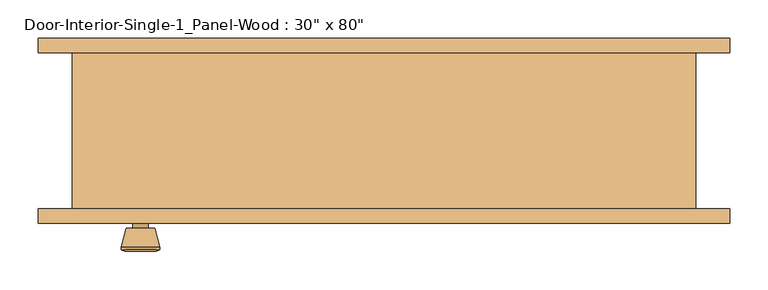
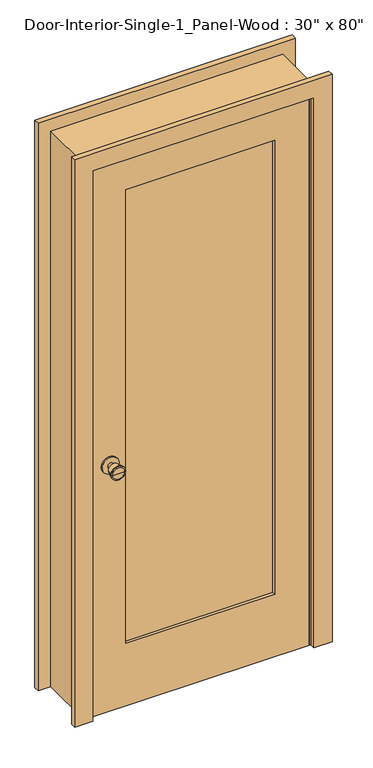
"""IFC4 building model written with IfcOpenShell, lengths in millimetres: door geometry."""

from ifc_helpers import new_model, si_unit, point, frame, frame_2d, origin, place, context, project, spatial, polyline, circle_curve, trimmed, segment, composite_curve, outline, extrude, faceted_brep, source, transform, mapped, element, save
from ifc_brep_helpers import plane_surface, cylinder_surface, revolved_surface, advanced_brep


def door_975671f7(model_context):
    return source(origin(), model_context, "Body", "SolidModel", [
        advanced_brep(
        [(-317.5, -57.5, 914.4), (-327.5, -57.5, 914.4), (-307.5, -57.5, 914.4), (-297.0241324, -8.5, 914.4), (-337.9758676, -8.5, 914.4), (-317.5, -8.5, 914.4), (-292.5, -10.3278681, 914.4), (-342.5, -10.3278681, 914.4), (-292.5, -13.7915463, 914.4), (-342.5, -13.7915463, 914.4), (-298.863764, -38.5, 914.4), (-336.136236, -38.5, 914.4), (-307.5, -38.5, 914.4), (-327.5, -38.5, 914.4)],
        [
            (0, 1),
            (1, 2, circle_curve(frame((-317.5, -57.5, 914.4), z_axis=(0.0, -1.0, 0.0), x_axis=(-1.0, 0.0, 0.0)), 10.0)),
            (2, 0),
            (2, 1, circle_curve(frame((-317.5, -57.5, 914.4), z_axis=(0.0, -1.0, 0.0), x_axis=(-1.0, 0.0, 0.0)), 10.0)),
            (3, 4, circle_curve(frame((-317.5, -8.5, 914.4), z_axis=(0.0, 1.0, 0.0), x_axis=(-1.0, 0.0, 0.0)), 20.4758676)),
            (4, 5),
            (5, 3),
            (4, 3, circle_curve(frame((-317.5, -8.5, 914.4), z_axis=(0.0, 1.0, 0.0), x_axis=(-1.0, 0.0, 0.0)), 20.4758676)),
            (6, 7, circle_curve(frame((-317.5, -10.3278681, 914.4), z_axis=(0.0, 1.0, 0.0), x_axis=(-1.0, 0.0, 0.0)), 25.0)),
            (7, 4),
            (3, 6),
            (7, 6, circle_curve(frame((-317.5, -10.3278681, 914.4), z_axis=(0.0, 1.0, 0.0), x_axis=(-1.0, 0.0, 0.0)), 25.0)),
            (8, 9, circle_curve(frame((-317.5, -13.7915463, 914.4), z_axis=(0.0, 1.0, 0.0), x_axis=(-1.0, 0.0, 0.0)), 25.0)),
            (9, 7),
            (6, 8),
            (9, 8, circle_curve(frame((-317.5, -13.7915463, 914.4), z_axis=(0.0, 1.0, 0.0), x_axis=(-1.0, 0.0, 0.0)), 25.0)),
            (10, 11, circle_curve(frame((-317.5, -38.5, 914.4), z_axis=(0.0, 1.0, 0.0), x_axis=(-1.0, 0.0, 0.0)), 18.636236)),
            (11, 9),
            (8, 10),
            (11, 10, circle_curve(frame((-317.5, -38.5, 914.4), z_axis=(0.0, 1.0, 0.0), x_axis=(-1.0, 0.0, 0.0)), 18.636236)),
            (12, 13, circle_curve(frame((-317.5, -38.5, 914.4), z_axis=(0.0, 1.0, 0.0), x_axis=(-1.0, 0.0, 0.0)), 10.0)),
            (13, 11),
            (10, 12),
            (13, 12, circle_curve(frame((-317.5, -38.5, 914.4), z_axis=(0.0, 1.0, 0.0), x_axis=(-1.0, 0.0, 0.0)), 10.0)),
            (1, 13),
            (12, 2),
        ],
        [
            plane_surface(frame((-317.5, -57.5, 914.4), z_axis=(0.0, -1.0, 0.0), x_axis=(-1.0, 0.0, 0.0))),
            plane_surface(frame((-317.5, -8.5, 914.4), z_axis=(0.0, 1.0, 0.0), x_axis=(-1.0, 0.0, 0.0))),
            revolved_surface(polyline([(-337.9758676, -8.5, 914.4), (-342.5, -10.3278681, 914.4)]), (-317.5, -57.5, 914.4), (0.0, -1.0, 0.0)),
            cylinder_surface(frame((-317.5, -57.5, 914.4), z_axis=(0.0, -1.0, 0.0), x_axis=(-1.0, 0.0, 0.0)), 25.0),
            revolved_surface(polyline([(-342.5, -13.7915463, 914.4), (-336.136236, -38.5, 914.4)]), (-317.5, -57.5, 914.4), (0.0, -1.0, 0.0)),
            plane_surface(frame((-317.5, -38.5, 914.4), z_axis=(0.0, -1.0, 0.0), x_axis=(-1.0, 0.0, 0.0))),
            cylinder_surface(frame((-317.5, -57.5, 914.4), z_axis=(0.0, -1.0, 0.0), x_axis=(-1.0, 0.0, 0.0)), 10.0),
        ],
        [
            (0, [[1, 2, 3]]),
            (0, [[-3, 4, -1]]),
            (1, [[5, 6, 7]]),
            (1, [[8, -7, -6]]),
            (2, [[9, 10, -5, 11]]),
            (2, [[12, -11, -8, -10]]),
            (3, [[13, 14, -9, 15]]),
            (3, [[16, -15, -12, -14]]),
            (4, [[17, 18, -13, 19]]),
            (4, [[20, -19, -16, -18]]),
            (5, [[21, 22, -17, 23]]),
            (5, [[24, -23, -20, -22]]),
            (6, [[-2, 25, -21, 26]]),
            (6, [[-4, -26, -24, -25]]),
        ],
    ),
        extrude(outline(composite_curve([segment(trimmed(circle_curve(frame_2d((914.4, -317.5)), 30.0), [point((914.4, -347.5))], [point((914.4, -287.5))], False, "CARTESIAN"), True, "CONTINUOUS"), segment(trimmed(circle_curve(frame_2d((914.4, -317.5)), 30.0), [point((914.4, -287.5))], [point((914.4, -347.5))], False, "CARTESIAN"), True, "CONTINUOUS")], self_intersect=False)), frame((0.0, -63.5, 0.0), z_axis=(0.0, 1.0, 0.0), x_axis=(0.0, 0.0, 1.0)), (0.0, 0.0, 1.0), 6.0),
        advanced_brep(
        [(-317.5, -104.425, 914.4), (-307.5, -104.425, 914.4), (-327.5, -104.425, 914.4), (-297.0241324, -153.425, 914.4), (-317.5, -153.425, 914.4), (-337.9758676, -153.425, 914.4), (-292.5, -151.5971319, 914.4), (-342.5, -151.5971319, 914.4), (-292.5, -148.1334537, 914.4), (-342.5, -148.1334537, 914.4), (-298.863764, -123.425, 914.4), (-336.136236, -123.425, 914.4), (-307.5, -123.425, 914.4), (-327.5, -123.425, 914.4)],
        [
            (0, 1),
            (1, 2, circle_curve(frame((-317.5, -104.425, 914.4), z_axis=(0.0, 1.0, 0.0), x_axis=(-1.0, 0.0, 0.0)), 10.0)),
            (2, 0),
            (2, 1, circle_curve(frame((-317.5, -104.425, 914.4), z_axis=(0.0, 1.0, 0.0), x_axis=(-1.0, 0.0, 0.0)), 10.0)),
            (3, 4),
            (4, 5),
            (5, 3, circle_curve(frame((-317.5, -153.425, 914.4), z_axis=(0.0, -1.0, 0.0), x_axis=(-1.0, 0.0, 0.0)), 20.4758676)),
            (3, 5, circle_curve(frame((-317.5, -153.425, 914.4), z_axis=(0.0, -1.0, 0.0), x_axis=(-1.0, 0.0, 0.0)), 20.4758676)),
            (6, 3),
            (5, 7),
            (7, 6, circle_curve(frame((-317.5, -151.5971319, 914.4), z_axis=(0.0, -1.0, 0.0), x_axis=(-1.0, 0.0, 0.0)), 25.0)),
            (6, 7, circle_curve(frame((-317.5, -151.5971319, 914.4), z_axis=(0.0, -1.0, 0.0), x_axis=(-1.0, 0.0, 0.0)), 25.0)),
            (8, 6),
            (7, 9),
            (9, 8, circle_curve(frame((-317.5, -148.1334537, 914.4), z_axis=(0.0, -1.0, 0.0), x_axis=(-1.0, 0.0, 0.0)), 25.0)),
            (8, 9, circle_curve(frame((-317.5, -148.1334537, 914.4), z_axis=(0.0, -1.0, 0.0), x_axis=(-1.0, 0.0, 0.0)), 25.0)),
            (10, 8),
            (9, 11),
            (11, 10, circle_curve(frame((-317.5, -123.425, 914.4), z_axis=(0.0, -1.0, 0.0), x_axis=(-1.0, 0.0, 0.0)), 18.636236)),
            (10, 11, circle_curve(frame((-317.5, -123.425, 914.4), z_axis=(0.0, -1.0, 0.0), x_axis=(-1.0, 0.0, 0.0)), 18.636236)),
            (12, 10),
            (11, 13),
            (13, 12, circle_curve(frame((-317.5, -123.425, 914.4), z_axis=(0.0, -1.0, 0.0), x_axis=(-1.0, 0.0, 0.0)), 10.0)),
            (12, 13, circle_curve(frame((-317.5, -123.425, 914.4), z_axis=(0.0, -1.0, 0.0), x_axis=(-1.0, 0.0, 0.0)), 10.0)),
            (1, 12),
            (13, 2),
        ],
        [
            plane_surface(frame((-317.5, -104.425, 914.4), z_axis=(0.0, 1.0, 0.0), x_axis=(-1.0, 0.0, 0.0))),
            plane_surface(frame((-317.5, -153.425, 914.4), z_axis=(0.0, -1.0, 0.0), x_axis=(-1.0, 0.0, 0.0))),
            revolved_surface(polyline([(-337.9758676, -153.425, 914.4), (-342.5, -151.5971319, 914.4)]), (-317.5, -104.425, 914.4), (0.0, 1.0, 0.0)),
            cylinder_surface(frame((-317.5, -104.425, 914.4), z_axis=(0.0, 1.0, 0.0), x_axis=(-1.0, 0.0, 0.0)), 25.0),
            revolved_surface(polyline([(-342.5, -148.1334537, 914.4), (-336.136236, -123.425, 914.4)]), (-317.5, -104.425, 914.4), (0.0, 1.0, 0.0)),
            plane_surface(frame((-317.5, -123.425, 914.4), z_axis=(0.0, 1.0, 0.0), x_axis=(-1.0, 0.0, 0.0))),
            cylinder_surface(frame((-317.5, -104.425, 914.4), z_axis=(0.0, 1.0, 0.0), x_axis=(-1.0, 0.0, 0.0)), 10.0),
        ],
        [
            (0, [[1, 2, 3]]),
            (0, [[-3, 4, -1]]),
            (1, [[5, 6, 7]]),
            (1, [[-6, -5, 8]]),
            (2, [[9, -7, 10, 11]]),
            (2, [[-10, -8, -9, 12]]),
            (3, [[13, -11, 14, 15]]),
            (3, [[-14, -12, -13, 16]]),
            (4, [[17, -15, 18, 19]]),
            (4, [[-18, -16, -17, 20]]),
            (5, [[21, -19, 22, 23]]),
            (5, [[-22, -20, -21, 24]]),
            (6, [[25, -23, 26, -2]]),
            (6, [[-26, -24, -25, -4]]),
        ],
    ),
        extrude(outline(composite_curve([segment(trimmed(circle_curve(frame_2d((914.4, -317.5)), 30.0), [point((914.4, -347.5))], [point((914.4, -287.5))], False, "CARTESIAN"), True, "CONTINUOUS"), segment(trimmed(circle_curve(frame_2d((914.4, -317.5)), 30.0), [point((914.4, -287.5))], [point((914.4, -347.5))], False, "CARTESIAN"), True, "CONTINUOUS")], self_intersect=False)), frame((0.0, -104.425, 0.0), z_axis=(0.0, 1.0, 0.0), x_axis=(0.0, 0.0, 1.0)), (0.0, 0.0, 1.0), 6.0),
        extrude(outline(polyline([(260.35, -75.1416667), (260.35, -86.7833333), (-260.35, -86.7833333), (-260.35, -75.1416667), (260.35, -75.1416667)])), frame((0.0, 0.0, 231.775), z_axis=(0.0, 0.0, 1.0), x_axis=(1.0, 0.0, 0.0)), (0.0, 0.0, 1.0), 1681.1625),
        extrude(outline(polyline([(2032.0, -381.0), (0.0, -381.0), (0.0, 381.0), (2032.0, 381.0), (2032.0, -381.0)]), holes=[polyline([(1912.9375, -260.35), (1912.9375, 260.35), (231.775, 260.35), (231.775, -260.35), (1912.9375, -260.35)])]), frame((0.0, -98.425, 0.0), z_axis=(0.0, 1.0, 0.0), x_axis=(0.0, 0.0, 1.0)), (0.0, 0.0, 1.0), 34.925),
        faceted_brep([(406.4, -98.425, 0.0), (381.0, -98.425, 0.0), (381.0, -63.5, 0.0), (368.3, -63.5, 0.0), (368.3, -28.575, 0.0), (381.0, -28.575, 0.0), (381.0, 104.775, 0.0), (406.4, 104.775, 0.0), (406.4, 104.775, 2057.4), (406.4, -98.425, 2057.4), (381.0, 104.775, 2032.0), (-381.0, 104.775, 2032.0), (-381.0, 104.775, 0.0), (-406.4, 104.775, 0.0), (-406.4, 104.775, 2057.4), (381.0, -28.575, 2032.0), (368.3, -28.575, 2019.3), (-368.3, -28.575, 2019.3), (-368.3, -28.575, 0.0), (-381.0, -28.575, 0.0), (-381.0, -28.575, 2032.0), (368.3, -63.5, 2019.3), (381.0, -63.5, 2032.0), (-381.0, -63.5, 2032.0), (-381.0, -63.5, 0.0), (-368.3, -63.5, 0.0), (-368.3, -63.5, 2019.3), (381.0, -98.425, 2032.0), (-406.4, -98.425, 2057.4), (-406.4, -98.425, 0.0), (-381.0, -98.425, 0.0), (-381.0, -98.425, 2032.0)], [[[0, 1, 2, 3, 4, 5, 6, 7]], [[7, 8, 9, 0]], [[6, 10, 11, 12, 13, 14, 8, 7]], [[5, 15, 10, 6]], [[4, 16, 17, 18, 19, 20, 15, 5]], [[3, 21, 16, 4]], [[2, 22, 23, 24, 25, 26, 21, 3]], [[1, 27, 22, 2]], [[0, 9, 28, 29, 30, 31, 27, 1]], [[8, 14, 28, 9]], [[15, 20, 11, 10]], [[21, 26, 17, 16]], [[27, 31, 23, 22]], [[29, 13, 12, 19, 18, 25, 24, 30]], [[14, 13, 29, 28]], [[20, 19, 12, 11]], [[26, 25, 18, 17]], [[31, 30, 24, 23]]]),
        extrude(outline(polyline([(0.0, 450.85), (2101.85, 450.85), (2101.85, -450.85), (0.0, -450.85), (0.0, -387.35), (2038.35, -387.35), (2038.35, 387.35), (0.0, 387.35), (0.0, 450.85)])), frame((0.0, 104.775, 0.0), z_axis=(0.0, 1.0, 0.0), x_axis=(0.0, 0.0, 1.0)), (0.0, 0.0, 1.0), 19.05),
        extrude(outline(polyline([(0.0, 450.85), (2101.85, 450.85), (2101.85, -450.85), (0.0, -450.85), (0.0, -387.35), (2038.35, -387.35), (2038.35, 387.35), (0.0, 387.35), (0.0, 450.85)])), frame((0.0, -117.475, 0.0), z_axis=(0.0, 1.0, 0.0), x_axis=(0.0, 0.0, 1.0)), (0.0, 0.0, 1.0), 19.05),
    ])


if __name__ == "__main__":
    model = new_model("IFC4")
    model_context = context("Model", 3, world=origin())
    ifc_project = project(units=[si_unit("LENGTHUNIT", "METRE", prefix="MILLI")], contexts=[model_context])
    site = spatial("IfcSite", under=ifc_project)
    building = spatial("IfcBuilding", under=site)
    placement = place(None, origin())
    door_shape = door_975671f7(model_context)
    element("IfcDoor", 1, ObjectType="Door-Interior-Single-1_Panel-Wood : 30\" x 80\"", at=placement, inside=building, context=model_context, shape_type="MappedRepresentation", body=[
        mapped(door_shape, transform((0.0, 0.0, 0.0), x_axis=(1.0, 0.0, 0.0), y_axis=(0.0, 1.0, 0.0), z_axis=(0.0, 0.0, 1.0))),
    ])
    save(model, "model.ifc")

# Revit data of these elements
# Type "Door-Interior-Single-1_Panel-Wood : 30\" x 80\""
#   Type Mark = "10"
#   Assembly Code = "C1020300"
#   Analytic Construction = "Wooden"
#   Top Rail = 0' - 4 11/16"
#   Thickness = 0' - 1 3/8"
#   Thermal Resistance (R) = 0.455703 (m²·K)/W
#   Swing Angle [instance default] = 90.00°
#   Stiles = 0' - 4 3/4"
#   Rough Width = 2' - 8"
#   Rough Height = 6' - 9"
#   Height = 6' - 8"
#   Width = 2' - 6"
#   Heat Transfer Coefficient (U) = 2.19465 W/(m²·K)
#   Bottom Rail = 0' - 9 1/8"
#   Trim Material = Cherry
#   Panel Material = Cherry
#   Frame Material = Cherry
#   Door Handle Material = Aluminum
#   Visual Light Transmittance = 0
#   Solar Heat Gain Coefficient = 0
#   Wall Closure = (empty or 0)
#   Function = (empty or 0)
# Element 1 (IfcDoor, "Door-Interior-Single-1_Panel-Wood : 30\" x 80\"")
#   Materials on its faces: "Cherry", "Aluminum"
# Materials
#   "Cherry": class "Wood", colour RGB 226 177 128, transparency 0, Description = "Prunus Serotina", Cost = 0
#   "Aluminum": class "Metal", colour RGB 247 247 247, transparency 0, Description = "Aluminum 6061", Cost = 0
